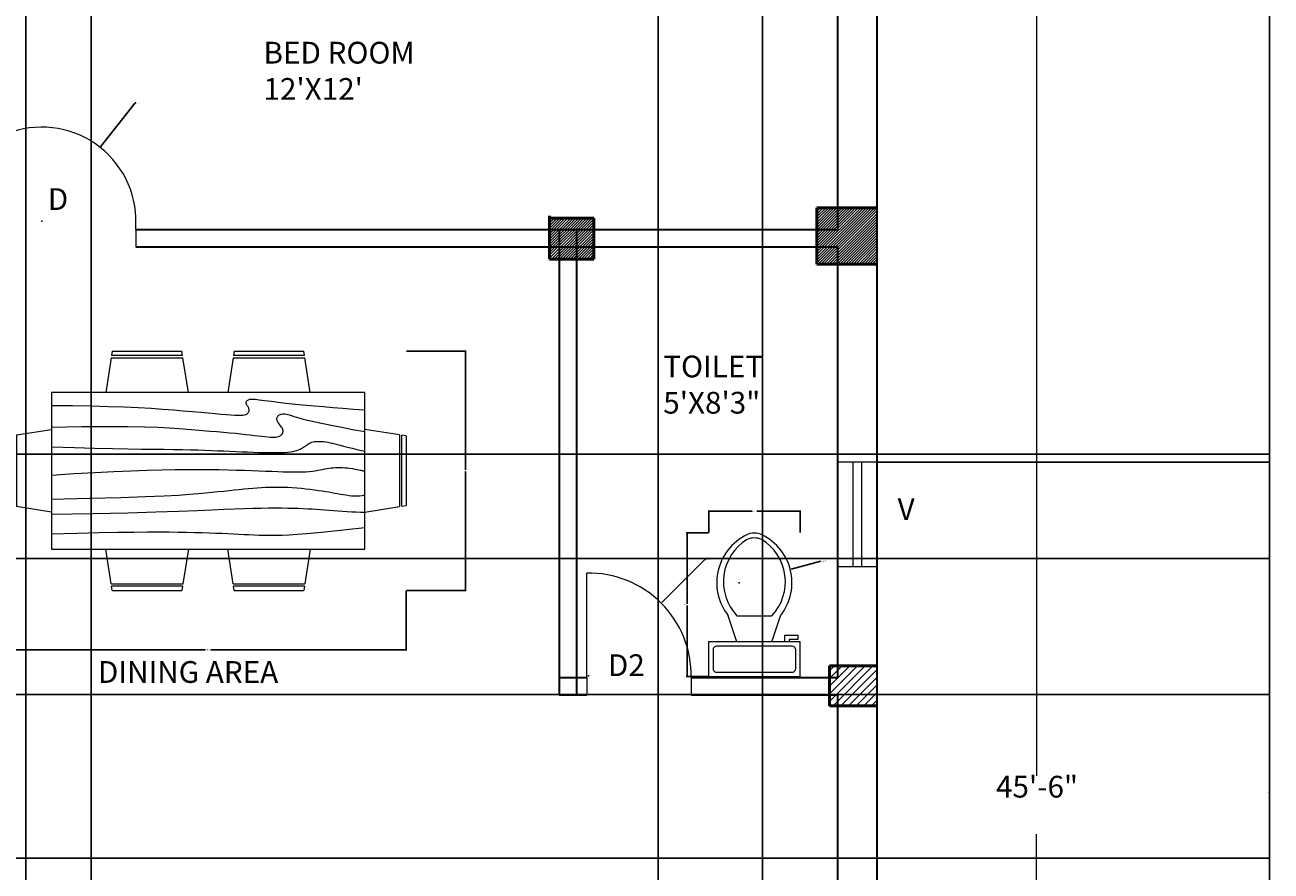
# Model space of a CAD drawing. Units: inches. Extents: x -12 to 472, y -585 to 99.
# Tile 3 of 4: x 186 to 472, y -281 to -86. Entities that reach past the tile are written whole.
import ezdxf

# ---------------------------------------------------------------- set-up
doc = ezdxf.new("R2010")
doc.units = ezdxf.units.IN
doc.header["$MEASUREMENT"] = 0
for name, color, linetype, lineweight in [('A-ANNO-DIMS', 2, 'Continuous', 18), ('A-ANNO-TEXT', 7, 'Continuous', 18), ('A-AREA-IDEN', 7, 'Continuous', 25), ('A-COLS', 7, 'Continuous', 50), ('A-COLS-PATT', 252, 'Continuous', 13), ('A-DOOR', 3, 'Continuous', 18), ('A-FLOR-FIXT', 9, 'Continuous', 20), ('A-FURN', 8, 'Continuous', 18), ('A-GLAZ', 4, 'Continuous', 18), ('A-WALL', 7, 'Continuous', 35)]:
    doc.layers.add(name, color=color, linetype=linetype, lineweight=lineweight)
doc.styles.get("Standard").update_dxf_attribs({"font": 'arial.ttf'})
doc.dimstyles.get("Standard").update_dxf_attribs({"dimtxt": 0.18, "dimasz": 0.18, "dimexe": 0.18, "dimexo": 0.0625, "dimgap": 0.09, "dimtad": 0, "dimtih": 1, "dimtoh": 1, "dimdec": 4, "dimzin": 0, "dimdsep": 46, "dimtxsty": 'Standard', "dimcen": 0.09, "dimadec": 0, "dimazin": 0, "dimtfac": 1, "dimtdec": 4, "dimtofl": 0, "dimtmove": 0, "dimatfit": 3, "dimfxl": 1, "dimtolj": 1, "dimtzin": 0, "dimarcsym": 0})

# ---------------------------------------------------------------- blocks, each defined once
blk = doc.blocks.new('Toilet - top')
for p, q in [((9.5, -6), (9.5, -2)), ((-10, -8.5), (-8, -8.5)), ((-10, -9.5), (-10, -8.5)), ((-8, -8.5), (-8, -8)), ((-7, -8), (-7, -9.5)), ((-4, -8), (-6, -14)), ((4, -8), (6, -14)), ((-7, -9.5), (-10, -9.5)), ((4, -14), (-4, -14))]:
    blk.add_line(p, q)
blk.add_lwpolyline([(10.5, -8), (10.5, 0), (-10.5, 0), (-10.5, -8)], close=True)
for points in [[(-9.5, -2), (-9.5, -6)], [(8.5, -1), (-8.5, -1)], [(-8.5, -7), (8.5, -7)]]:
    blk.add_lwpolyline(points)
for centre, radius, start, end in [((-8.62, -1.88), 0.884, 81.8699, 188.1301), ((8.62, -1.88), 0.884, 351.8699, 98.1301), ((-8.62, -6.12), 0.884, 171.8699, 278.1301), ((8.62, -6.12), 0.884, 261.8699, 8.1301), ((3.52, -21.58), 12.17, 141.4691, 247.9714), ((4.2, -21.82), 11.33, 136.3677, 238.9468), ((-3.52, -21.58), 12.17, 292.0284, 38.5307), ((-4.2, -21.82), 11.33, 301.053, 43.6321), ((0, -27.88), 4, 245.7318, 294.2682), ((0, -29), 4, 254.8605, 285.1395)]:
    blk.add_arc(centre, radius, start, end)
blk = doc.blocks.new('Dining Set - 36 x 72 in.')
for p, q in [((-22.2343, 26.00059), (-23.4847, 17.99762)), ((-22.2304, 26), (-5.7608, 26)), ((-22, 27.5), (-22.1562, 26.50042)), ((-5.8416, 26.5), (-22.1534, 26.5)), ((-22, 27.5), (-6, 27.5)), ((-5.8437, 26.49966), (-6, 27.5)), ((-4.5152, 17.99762), (-5.7655, 25.99926)), ((5.7657, 26.00059), (4.5153, 17.99762)), ((5.7696, 26), (22.2392, 26)), ((6, 27.5), (5.8438, 26.50042)), ((22.1584, 26.5), (5.8466, 26.5)), ((6, 27.5), (22, 27.5)), ((22.1563, 26.49966), (22, 27.5)), ((23.4848, 17.99762), (22.2345, 25.99926)), ((36, 18), (-36, 18)), ((-36, 18), (-36, -18)), ((36, -18), (36, 18)), ((-44.0006, 8.23428), (-35.9976, 9.48474)), ((44.0006, 8.23428), (35.9976, 9.48474)), ((-45.5, 8), (-44.5004, 8.15617)), ((-45.5, 8), (-45.5, -8)), ((-44.5, -8.15843), (-44.5, 8.15338)), ((-44, 8.23041), (-44, -8.23915)), ((44, 8.23041), (44, -8.23915)), ((44.5, -8.15843), (44.5, 8.15338)), ((45.5, 8), (44.5005, 8.15617)), ((45.5, 8), (45.5, -8)), ((-44.4997, -8.15631), (-45.5, -8)), ((-35.9976, -9.48476), (-43.9993, -8.2345)), ((35.9976, -9.48476), (43.9993, -8.2345)), ((44.4997, -8.15631), (45.5, -8)), ((-36, -18), (36, -18)), ((-22.2343, -26.0006), (-23.4847, -17.99762)), ((-4.5152, -17.99762), (-5.7655, -25.99928)), ((5.7657, -26.0006), (4.5153, -17.99762)), ((23.4848, -17.99762), (22.2345, -25.99928)), ((-22.2304, -26), (-5.7608, -26)), ((-22, -27.5), (-22.1562, -26.50044)), ((-5.8416, -26.5), (-22.1534, -26.5)), ((-22, -27.5), (-6, -27.5)), ((-5.8437, -26.49967), (-6, -27.5)), ((5.7696, -26), (22.2392, -26)), ((6, -27.5), (5.8438, -26.50044)), ((22.1584, -26.5), (5.8466, -26.5)), ((6, -27.5), (22, -27.5)), ((22.1563, -26.49967), (22, -27.5))]:
    blk.add_line(p, q)
for points in [[(-36, 15), (-31.1772, 14.97754), (-26.8079, 14.91406), (-22.8538, 14.81543), (-19.276, 14.6875), (-16.0362, 14.53613), (-13.0957, 14.36718), (-10.4159, 14.18652), (-7.9583, 14), (-5.6904, 13.81315), (-3.6035, 13.63021), (-1.6954, 13.45508), (0.0365, 13.29166), (1.5945, 13.14388), (2.9811, 13.01562), (4.1988, 12.9108), (5.25, 12.83333), (6.1393, 12.78613), (6.8802, 12.76823), (7.4883, 12.77767), (7.9792, 12.8125), (8.3685, 12.87077), (8.6719, 12.95052), (8.9049, 13.0498), (9.0833, 13.16666), (9.2205, 13.29899), (9.3216, 13.44401), (9.3895, 13.59879), (9.4271, 13.76041), (9.4373, 13.92594), (9.4232, 14.09245), (9.3875, 14.257), (9.3333, 14.41666), (9.2638, 14.56917), (9.1836, 14.71484), (9.0975, 14.85465), (9.0104, 14.98958), (8.9272, 15.1206), (8.8529, 15.2487), (8.7922, 15.37483), (8.75, 15.5), (8.7305, 15.62467), (8.7344, 15.74739), (8.7617, 15.86621), (8.8125, 15.97916), (8.8867, 16.08431), (8.9844, 16.17968), (9.1055, 16.26334), (9.25, 16.33333), (9.4189, 16.38802), (9.6172, 16.42708), (9.8506, 16.45052), (10.125, 16.45833), (10.4463, 16.45052), (10.8203, 16.42708), (11.2529, 16.38802), (11.75, 16.33333), (12.3184, 16.26318), (12.9694, 16.17838), (13.7151, 16.07991), (14.5677, 15.96875), (15.5395, 15.84586), (16.6426, 15.71224), (17.8893, 15.56884), (19.2917, 15.41666), (20.859, 15.25667), (22.5879, 15.08984), (24.4721, 14.91715), (26.5052, 14.73958), (28.6809, 14.5581), (30.9929, 14.3737), (33.4347, 14.18733), (36, 14)], [(-36, 10), (-28.9766, 10.14274), (-23.1725, 10.20442), (-18.4241, 10.19775), (-14.5677, 10.13541), (-11.4399, 10.03011), (-8.877, 9.89453), (-6.7154, 9.74137), (-4.7917, 9.58333), (-2.9698, 9.43082), (-1.2246, 9.28515), (0.4415, 9.14534), (2.026, 9.01041), (3.5266, 8.87939), (4.9408, 8.7513), (6.266, 8.62516), (7.5, 8.5), (8.6411, 8.37549), (9.6914, 8.2539), (10.6538, 8.13818), (11.5312, 8.03125), (12.3267, 7.93603), (13.043, 7.85547), (13.6831, 7.79248), (14.25, 7.75), (14.7471, 7.7303), (15.1797, 7.73307), (15.5537, 7.75732), (15.875, 7.80208), (16.1494, 7.86637), (16.3828, 7.94922), (16.5811, 8.04964), (16.75, 8.16666), (16.8944, 8.29915), (17.0143, 8.44531), (17.1089, 8.60319), (17.1771, 8.77083), (17.218, 8.94629), (17.2305, 9.1276), (17.2137, 9.31282), (17.1667, 9.5), (17.0895, 9.6875), (16.987, 9.875), (16.8649, 10.0625), (16.7292, 10.25), (16.5856, 10.4375), (16.4401, 10.625), (16.2985, 10.8125), (16.1667, 11), (16.05, 11.18733), (15.9518, 11.3737), (15.8752, 11.5581), (15.8229, 11.73958), (15.798, 11.91715), (15.8034, 12.08984), (15.842, 12.25667), (15.9167, 12.41666), (16.0295, 12.56836), (16.1784, 12.70833), (16.3605, 12.83268), (16.5729, 12.9375), (16.8127, 13.01888), (17.0768, 13.07291), (17.3625, 13.0957), (17.6667, 13.08333), (17.9894, 13.03312), (18.3418, 12.94726), (18.7382, 12.82918), (19.1927, 12.68229), (19.7195, 12.51001), (20.3327, 12.31575), (21.0465, 12.10294), (21.875, 11.875), (22.8357, 11.63354), (23.959, 11.37304), (25.2786, 11.08618), (26.8282, 10.76562), (28.6414, 10.40405), (30.752, 9.99414), (33.1936, 9.52856), (36, 9)], [(-36, 5.5), (-30.7157, 5.3348), (-26.069, 5.20963), (-21.9946, 5.11767), (-18.4271, 5.05208), (-15.3009, 5.00602), (-12.5508, 4.97265), (-10.1112, 4.94515), (-7.9167, 4.91666), (-5.909, 4.88167), (-4.0586, 4.83984), (-2.3429, 4.79215), (-0.7396, 4.73958), (0.7739, 4.6831), (2.22, 4.6237), (3.6213, 4.56233), (5, 4.5), (6.373, 4.43782), (7.7344, 4.3776), (9.0723, 4.32129), (10.375, 4.27083), (11.6309, 4.22819), (12.8281, 4.19531), (13.9551, 4.17415), (15, 4.16666), (15.954, 4.17448), (16.819, 4.19791), (17.6001, 4.23698), (18.3021, 4.29166), (18.9299, 4.36198), (19.4883, 4.44791), (19.9823, 4.54948), (20.4167, 4.66666), (20.7969, 4.79899), (21.1302, 4.94401), (21.4245, 5.09879), (21.6875, 5.26041), (21.9271, 5.42594), (22.1511, 5.59245), (22.3672, 5.757), (22.5834, 5.91666), (22.8065, 6.06868), (23.0404, 6.21093), (23.2879, 6.34147), (23.5521, 6.45833), (23.8358, 6.55957), (24.142, 6.64323), (24.4735, 6.70735), (24.8334, 6.75), (25.2235, 6.76969), (25.642, 6.76692), (26.0858, 6.74267), (26.5521, 6.69791), (27.0379, 6.63362), (27.5404, 6.55078), (28.0565, 6.45036), (28.5834, 6.33333), (29.1242, 6.19987), (29.7071, 6.04687), (30.3661, 5.87044), (31.1354, 5.66666), (32.0493, 5.43164), (33.142, 5.16146), (34.4475, 4.85221), (36, 4.5)], [(-36, -1), (-30.7915, -0.6591), (-26.0195, -0.38216), (-21.6519, -0.16284), (-17.6563, 0.00521), (-14.0005, 0.12833), (-10.6523, 0.21289), (-7.5796, 0.26522), (-4.75, 0.29166), (-2.134, 0.29793), (0.2878, 0.28711), (2.5317, 0.26163), (4.6146, 0.22396), (6.5529, 0.17651), (8.3633, 0.12174), (10.0623, 0.06209), (11.6667, 0), (13.1899, -0.06201), (14.6341, -0.1211), (15.9982, -0.17432), (17.2813, -0.21875), (18.4823, -0.25147), (19.6003, -0.26953), (20.6343, -0.27002), (21.5834, -0.25), (22.4481, -0.20768), (23.2357, -0.14584), (23.9549, -0.06836), (24.6146, 0.02083), (25.2235, 0.11784), (25.7904, 0.21875), (26.3241, 0.31966), (26.8334, 0.41666), (27.3265, 0.50618), (27.8099, 0.58593), (28.2894, 0.65397), (28.7709, 0.70833), (29.2601, 0.74707), (29.763, 0.76823), (30.2855, 0.76985), (30.8334, 0.75), (31.4088, 0.70784), (31.9994, 0.64713), (32.589, 0.57275), (33.1615, 0.48958), (33.7008, 0.4025), (34.1908, 0.3164), (34.6153, 0.23616), (34.9584, 0.16666), (35.2099, 0.11165), (35.3848, 0.07031), (35.504, 0.04069), (35.5886, 0.02083), (35.6594, 0.00879), (35.7377, 0.0026), (35.8442, 0.00032), (36, 0)], [(-36, -6.5), (-27.1843, -6.31267), (-20.084, -6.1263), (-14.469, -5.9419), (-10.1094, -5.76042), (-6.7752, -5.58285), (-4.2363, -5.41016), (-2.2629, -5.24333), (-0.625, -5.08334), (0.8708, -4.93099), (2.2715, -4.78646), (3.5872, -4.64974), (4.8281, -4.52084), (6.0046, -4.39974), (7.127, -4.28646), (8.2053, -4.18099), (9.25, -4.08334), (10.2705, -3.99382), (11.2734, -3.91407), (12.2647, -3.84603), (13.25, -3.79167), (14.2354, -3.75293), (15.2266, -3.73177), (16.2295, -3.73015), (17.25, -3.75), (18.2912, -3.79248), (19.3451, -3.85547), (20.4009, -3.93604), (21.4479, -4.03125), (22.4754, -4.13819), (23.4727, -4.25391), (24.4289, -4.37549), (25.3334, -4.5), (26.1785, -4.62492), (26.9694, -4.74935), (27.7145, -4.87281), (28.4219, -4.99479), (29.1, -5.11483), (29.7572, -5.23242), (30.4016, -5.34709), (31.0417, -5.45834), (31.6837, -5.56437), (32.3262, -5.65821), (32.9658, -5.73153), (33.599, -5.77604), (34.2224, -5.78345), (34.8327, -5.74545), (35.4264, -5.65373), (36, -5.5)], [(-36, -10), (-26.4022, -9.81299), (-18.4675, -9.62891), (-11.9839, -9.45069), (-6.7396, -9.28125), (-2.5226, -9.12354), (0.8789, -8.98047), (3.6769, -8.85498), (6.0833, -8.75), (8.2767, -8.66765), (10.3021, -8.60677), (12.1712, -8.56543), (13.8958, -8.54167), (15.4876, -8.53353), (16.9583, -8.53907), (18.3197, -8.55632), (19.5834, -8.58334), (20.7616, -8.61841), (21.8685, -8.66081), (22.9188, -8.71004), (23.9271, -8.76563), (24.9081, -8.82707), (25.8763, -8.89388), (26.8465, -8.96558), (27.8334, -9.04167), (28.8474, -9.12118), (29.8828, -9.20117), (30.93, -9.27824), (31.9792, -9.34896), (33.0205, -9.40991), (34.0443, -9.45768), (35.0407, -9.48885), (36, -9.5)], [(-36, -14.5), (-30.0881, -14.33513), (-25.0332, -14.21224), (-20.7312, -14.12647), (-17.0781, -14.07292), (-13.97, -14.04671), (-11.3027, -14.04297), (-8.9724, -14.05681), (-6.875, -14.08334), (-4.9224, -14.11833), (-3.0905, -14.16016), (-1.3709, -14.20785), (0.2448, -14.26042), (1.7647, -14.3169), (3.1973, -14.3763), (4.5507, -14.43767), (5.8333, -14.5), (7.0554, -14.5621), (8.235, -14.62175), (9.3922, -14.67652), (10.5469, -14.72396), (11.7192, -14.76164), (12.929, -14.78711), (14.1965, -14.79794), (15.5417, -14.79167), (16.9933, -14.76424), (18.6152, -14.70508), (20.4804, -14.60197), (22.6615, -14.44271), (25.2312, -14.21509), (28.2624, -13.9069), (31.8277, -13.50594), (36, -13)]]:
    blk.add_lwpolyline(points)
blk = doc.blocks.new('VENT-24IN-EXT')
for p, q in [((0, 5.5), (24, 5.5)), ((0, 3.5), (24, 3.5))]:
    blk.add_line(p, q)
blk.add_lwpolyline([(0, 9), (24, 9), (24, 0), (0, 0)], close=True)
blk = doc.blocks.new('*D20')
at = {"layer": 'A-ANNO-DIMS', "color": 0, "lineweight": -2, "transparency": 16777216}
for p, q in [((342.6, -203.13), (337.52, -203.13)), ((337.7, -203.31), (337.7, -219.47)), ((337.7, -236), (337.7, -219.84)), ((342.6, -236.18), (337.52, -236.18))]:
    blk.add_line(p, q, dxfattribs=at)
at = {"layer": 'A-ANNO-DIMS', "color": 0, "transparency": 16777216}
for points in [[(337.67, -203.31), (337.73, -203.31), (337.7, -203.13)], [(337.67, -236), (337.73, -236), (337.7, -236.18)]]:
    blk.add_solid(points, dxfattribs=at)
at = {"layer": 'Defpoints', "color": 0, "transparency": 16777216}
for p in [(342.66, -203.13), (337.7, -236.18), (342.66, -236.18)]:
    blk.add_point(p, dxfattribs=at)
at = {"layer": 'A-ANNO-DIMS', "color": 0, "transparency": 16777216, "insert": (337.7, -219.66), "char_height": 0.18, "attachment_point": 5}
blk.add_mtext('\\A1;WC 33 TYP.', dxfattribs=at)
blk = doc.blocks.new('*D21')
at = {"layer": 'A-ANNO-DIMS', "color": 0, "lineweight": -2, "transparency": 16777216}
for p, q in [((342.66, -203.07), (342.66, -198)), ((342.84, -198.18), (352.63, -198.18)), ((363.48, -198.18), (353.69, -198.18)), ((363.66, -203.07), (363.66, -198))]:
    blk.add_line(p, q, dxfattribs=at)
at = {"layer": 'A-ANNO-DIMS', "color": 0, "transparency": 16777216}
for points in [[(342.84, -198.15), (342.84, -198.21), (342.66, -198.18)], [(363.48, -198.15), (363.48, -198.21), (363.66, -198.18)]]:
    blk.add_solid(points, dxfattribs=at)
at = {"layer": 'Defpoints', "color": 0, "transparency": 16777216}
for p in [(342.66, -198.18), (342.66, -203.13), (363.66, -203.13)]:
    blk.add_point(p, dxfattribs=at)
at = {"layer": 'A-ANNO-DIMS', "color": 0, "transparency": 16777216, "insert": (353.16, -198.18), "char_height": 0.18, "attachment_point": 5}
blk.add_mtext('\\A1;21 TYP.', dxfattribs=at)
blk = doc.blocks.new('*D24')
at = {"layer": 'A-ANNO-DIMS', "color": 0, "lineweight": -2, "transparency": 16777216}
for p, q in [((182.14, -216.43), (182.14, -230.2)), ((273.14, -216.43), (273.14, -230.2)), ((182.32, -230.02), (226.97, -230.02)), ((272.96, -230.02), (228.31, -230.02))]:
    blk.add_line(p, q, dxfattribs=at)
at = {"layer": 'A-ANNO-DIMS', "color": 0, "transparency": 16777216}
for points in [[(182.32, -229.99), (182.32, -230.05), (182.14, -230.02)], [(272.96, -229.99), (272.96, -230.05), (273.14, -230.02)]]:
    blk.add_solid(points, dxfattribs=at)
at = {"layer": 'Defpoints', "color": 0, "transparency": 16777216}
for p in [(182.14, -216.37), (273.14, -216.37), (273.14, -230.02)]:
    blk.add_point(p, dxfattribs=at)
at = {"layer": 'A-ANNO-DIMS', "color": 0, "transparency": 16777216, "insert": (227.64, -230.02), "char_height": 0.18, "attachment_point": 5}
blk.add_mtext('\\A1;DINING 91', dxfattribs=at)
blk = doc.blocks.new('*D25')
at = {"layer": 'A-ANNO-DIMS', "color": 0, "lineweight": -2, "transparency": 16777216}
for p, q in [((273.2, -161.37), (286.97, -161.37)), ((286.79, -161.55), (286.79, -188.68)), ((286.79, -216.19), (286.79, -189.05)), ((273.2, -216.37), (286.97, -216.37))]:
    blk.add_line(p, q, dxfattribs=at)
at = {"layer": 'A-ANNO-DIMS', "color": 0, "transparency": 16777216}
for points in [[(286.76, -161.55), (286.82, -161.55), (286.79, -161.37)], [(286.76, -216.19), (286.82, -216.19), (286.79, -216.37)]]:
    blk.add_solid(points, dxfattribs=at)
at = {"layer": 'Defpoints', "color": 0, "transparency": 16777216}
for p in [(273.14, -161.37), (286.79, -161.37), (273.14, -216.37)]:
    blk.add_point(p, dxfattribs=at)
at = {"layer": 'A-ANNO-DIMS', "color": 0, "transparency": 16777216, "insert": (286.79, -188.87), "char_height": 0.18, "attachment_point": 5}
blk.add_mtext('\\A1;55', dxfattribs=at)
blk = doc.blocks.new('*D30')
at = {"layer": 'A-ANNO-DIMS', "color": 0, "lineweight": -2, "transparency": 16777216}
for p, q in [((185.8, -429.83), (185.8, 98.81)), ((185.98, 98.63), (193.09, 98.63)), ((200.62, 98.63), (193.51, 98.63)), ((200.8, -431.32), (200.8, 98.81))]:
    blk.add_line(p, q, dxfattribs=at)
at = {"layer": 'A-ANNO-DIMS', "color": 0, "transparency": 16777216}
for points in [[(185.98, 98.66), (185.98, 98.6), (185.8, 98.63)], [(200.62, 98.66), (200.62, 98.6), (200.8, 98.63)]]:
    blk.add_solid(points, dxfattribs=at)
at = {"layer": 'Defpoints', "color": 0, "transparency": 16777216}
for p in [(200.8, 98.63), (185.8, -429.9), (200.8, -431.38)]:
    blk.add_point(p, dxfattribs=at)
at = {"layer": 'A-ANNO-DIMS', "color": 0, "transparency": 16777216, "insert": (193.3, 98.63), "char_height": 0.18, "attachment_point": 5}
blk.add_mtext('\\A1;15', dxfattribs=at)
blk = doc.blocks.new('*D37')
at = {"layer": 'A-ANNO-DIMS', "color": 0, "lineweight": -2, "transparency": 16777216}
for p, q in [((138.68, -240.32), (471.69, -240.32)), ((471.51, -240.5), (471.51, -258.92)), ((471.51, -277.7), (471.51, -259.28)), ((138.68, -277.88), (471.69, -277.88))]:
    blk.add_line(p, q, dxfattribs=at)
at = {"layer": 'A-ANNO-DIMS', "color": 0, "transparency": 16777216}
for points in [[(471.48, -240.5), (471.54, -240.5), (471.51, -240.32)], [(471.48, -277.7), (471.54, -277.7), (471.51, -277.88)]]:
    blk.add_solid(points, dxfattribs=at)
at = {"layer": 'Defpoints', "color": 0, "transparency": 16777216}
for p in [(138.61, -240.32), (138.61, -277.88), (471.51, -277.88)]:
    blk.add_point(p, dxfattribs=at)
at = {"layer": 'A-ANNO-DIMS', "color": 0, "transparency": 16777216, "insert": (471.51, -259.1), "char_height": 0.18, "attachment_point": 5}
blk.add_mtext('\\A1;37.56', dxfattribs=at)
blk = doc.blocks.new('*D40')
at = {"layer": 'A-ANNO-DIMS', "color": 0, "lineweight": -2, "transparency": 16777216}
for p, q in [((331.04, -77.44), (331.04, -585.26)), ((355.04, -77.44), (355.04, -585.26)), ((331.22, -585.08), (342.82, -585.08)), ((354.86, -585.08), (343.26, -585.08))]:
    blk.add_line(p, q, dxfattribs=at)
at = {"layer": 'A-ANNO-DIMS', "color": 0, "transparency": 16777216}
for points in [[(331.22, -585.05), (331.22, -585.11), (331.04, -585.08)], [(354.86, -585.05), (354.86, -585.11), (355.04, -585.08)]]:
    blk.add_solid(points, dxfattribs=at)
at = {"layer": 'Defpoints', "color": 0, "transparency": 16777216}
for p in [(331.04, -77.38), (355.04, -77.38), (355.04, -585.08)]:
    blk.add_point(p, dxfattribs=at)
at = {"layer": 'A-ANNO-DIMS', "color": 0, "transparency": 16777216, "insert": (343.04, -585.08), "char_height": 0.18, "attachment_point": 5}
blk.add_mtext('\\A1;24', dxfattribs=at)
blk = doc.blocks.new('*D46')
at = {"layer": 'A-ANNO-DIMS', "color": 0, "lineweight": -2, "transparency": 16777216}
for p, q in [((133.34, -185.05), (471.69, -185.05)), ((471.51, -185.23), (471.51, -196.87)), ((471.51, -208.87), (471.51, -197.23)), ((133.34, -209.05), (471.69, -209.05))]:
    blk.add_line(p, q, dxfattribs=at)
at = {"layer": 'A-ANNO-DIMS', "color": 0, "transparency": 16777216}
for points in [[(471.48, -185.23), (471.54, -185.23), (471.51, -185.05)], [(471.48, -208.87), (471.54, -208.87), (471.51, -209.05)]]:
    blk.add_solid(points, dxfattribs=at)
at = {"layer": 'Defpoints', "color": 0, "transparency": 16777216}
for p in [(133.28, -185.05), (133.28, -209.05), (471.51, -209.05)]:
    blk.add_point(p, dxfattribs=at)
at = {"layer": 'A-ANNO-DIMS', "color": 0, "transparency": 16777216, "insert": (471.51, -197.05), "char_height": 0.18, "attachment_point": 5}
blk.add_mtext('\\A1;24', dxfattribs=at)
blk = doc.blocks.new('*D50')
at = {"layer": 'A-ANNO-DIMS', "color": 0, "lineweight": -2, "transparency": 16777216}
for p, q in [((381.34, 19.62), (471.69, 19.62)), ((471.51, 19.44), (471.51, -83.45)), ((471.51, -186.7), (471.51, -83.81)), ((381.34, -186.88), (471.69, -186.88))]:
    blk.add_line(p, q, dxfattribs=at)
at = {"layer": 'A-ANNO-DIMS', "color": 0, "transparency": 16777216}
for points in [[(471.48, 19.44), (471.54, 19.44), (471.51, 19.62)], [(471.48, -186.7), (471.54, -186.7), (471.51, -186.88)]]:
    blk.add_solid(points, dxfattribs=at)
at = {"layer": 'Defpoints', "color": 0, "transparency": 16777216}
for p in [(381.28, 19.62), (381.28, -186.88), (471.51, -186.88)]:
    blk.add_point(p, dxfattribs=at)
at = {"layer": 'A-ANNO-DIMS', "color": 0, "transparency": 16777216, "insert": (471.51, -83.63), "char_height": 0.18, "attachment_point": 5}
blk.add_mtext('\\A1;206.5', dxfattribs=at)
blk = doc.blocks.new('*D51')
at = {"layer": 'A-ANNO-DIMS', "color": 0, "lineweight": -2, "transparency": 16777216}
for p, q in [((381.34, -186.88), (471.69, -186.88)), ((471.51, -187.06), (471.51, -262.66)), ((471.51, -338.62), (471.51, -263.02)), ((381.34, -338.8), (471.69, -338.8))]:
    blk.add_line(p, q, dxfattribs=at)
at = {"layer": 'A-ANNO-DIMS', "color": 0, "transparency": 16777216}
for points in [[(471.48, -187.06), (471.54, -187.06), (471.51, -186.88)], [(471.48, -338.62), (471.54, -338.62), (471.51, -338.8)]]:
    blk.add_solid(points, dxfattribs=at)
at = {"layer": 'Defpoints', "color": 0, "transparency": 16777216}
for p in [(381.28, -186.88), (381.28, -338.8), (471.51, -338.8)]:
    blk.add_point(p, dxfattribs=at)
at = {"layer": 'A-ANNO-DIMS', "color": 0, "transparency": 16777216, "insert": (471.51, -262.84), "char_height": 0.18, "attachment_point": 5}
blk.add_mtext('\\A1;151.92', dxfattribs=at)
blk = doc.blocks.new('*D57')
at = {"layer": 'A-ANNO-DIMS', "color": 0, "lineweight": -2, "transparency": 16777216}
for p, q in [((341.76, -209.28), (331.87, -219.16)), ((341.94, -209.28), (341.76, -209.28)), ((314.98, -235.97), (315.16, -235.97)), ((315.07, -236.06), (315.07, -235.88))]:
    blk.add_line(p, q, dxfattribs=at)
at = {"layer": 'A-ANNO-DIMS', "color": 0, "transparency": 16777216}
blk.add_solid([(331.85, -219.14), (331.9, -219.18), (331.75, -219.28)], dxfattribs=at)
at = {"layer": 'Defpoints', "color": 0, "transparency": 16777216}
for p in [(331.75, -219.28), (315.07, -235.97)]:
    blk.add_point(p, dxfattribs=at)
at = {"layer": 'A-ANNO-DIMS', "color": 0, "transparency": 16777216, "insert": (342.42, -209.28), "char_height": 0.18, "attachment_point": 5}
blk.add_mtext('\\A1;R23.59', dxfattribs=at)
blk = doc.blocks.new('*D58')
at = {"layer": 'A-ANNO-DIMS', "color": 0, "lineweight": -2, "transparency": 16777216}
for p, q in [((210.88, -104.32), (202.95, -114.38)), ((211.06, -104.32), (210.88, -104.32)), ((189.35, -131.51), (189.53, -131.51)), ((189.44, -131.6), (189.44, -131.42))]:
    blk.add_line(p, q, dxfattribs=at)
at = {"layer": 'A-ANNO-DIMS', "color": 0, "transparency": 16777216}
blk.add_solid([(202.93, -114.36), (202.98, -114.39), (202.84, -114.52)], dxfattribs=at)
at = {"layer": 'Defpoints', "color": 0, "transparency": 16777216}
for p in [(202.84, -114.52), (189.44, -131.51)]:
    blk.add_point(p, dxfattribs=at)
at = {"layer": 'A-ANNO-DIMS', "color": 0, "transparency": 16777216, "insert": (211.61, -104.32), "char_height": 0.18, "attachment_point": 5}
blk.add_mtext('\\A1;R21.644', dxfattribs=at)
blk = doc.blocks.new('*D62')
at = {"layer": 'A-ANNO-DIMS', "color": 0, "lineweight": -2, "transparency": 16777216}
for p, q in [((368.47, -209.65), (361.58, -211.46)), ((349.55, -214.6), (349.73, -214.6)), ((349.64, -214.69), (349.64, -214.51))]:
    blk.add_line(p, q, dxfattribs=at)
at = {"layer": 'A-ANNO-DIMS', "color": 0, "transparency": 16777216}
blk.add_solid([(361.58, -211.43), (361.59, -211.49), (361.41, -211.51)], dxfattribs=at)
at = {"layer": 'Defpoints', "color": 0, "transparency": 16777216}
for p in [(361.41, -211.51), (349.64, -214.6)]:
    blk.add_point(p, dxfattribs=at)
at = {"layer": 'A-ANNO-DIMS', "color": 0, "transparency": 16777216, "insert": (369.15, -209.65), "char_height": 0.18, "attachment_point": 5}
blk.add_mtext('\\A1;4X R12.17', dxfattribs=at)

msp = doc.modelspace()

# ---------------------------------------------------------------- hatches: boundary and pattern name
at = {"layer": 'A-COLS-PATT'}
h = msp.add_hatch(dxfattribs=at)
h.set_pattern_fill('ANSI31', color=256, scale=3.5)
h.set_pattern_definition([(45, (-1281.90016, -702.76037), (-0.30935922, 0.30935922), [])])
h.paths.add_polyline_path([(178.2783, -133.3788), (174.2783, -133.3788), (174.2783, -137.3788), (178.2783, -137.3788)])
h.paths.add_polyline_path([(178.2783, -130.763), (174.2783, -130.763), (174.2783, -133.3788), (178.2783, -133.3788)])
h.paths.add_polyline_path([(174.2783, -130.763), (172.7504, -130.763), (172.7504, -133.3788), (174.2783, -133.3788)])
h.paths.add_polyline_path([(174.2783, -133.3788), (172.7504, -133.3788), (172.7504, -137.3788), (174.2783, -137.3788)])
h.paths.add_polyline_path([(181.0026, -137.3788), (172.7504, -137.3788), (172.7504, -139.195), (181.0026, -139.195)])
h.paths.add_polyline_path([(181.0026, -133.3788), (178.2783, -133.3788), (178.2783, -137.3788), (181.0026, -137.3788)])
h.paths.add_polyline_path([(181.0026, -130.763), (178.2783, -130.763), (178.2783, -133.3788), (181.0026, -133.3788)])
h.paths.add_polyline_path([(381.2783, -128.4288), (372.2783, -128.4288), (372.2783, -133.3788), (367.5282, -133.3788), (367.5282, -137.3788), (372.2783, -137.3788), (372.2783, -141.3418), (381.2783, -141.3418)])
h.paths.add_polyline_path([(372.2783, -128.4288), (367.5282, -128.4288), (367.5282, -133.3788), (372.2783, -133.3788)])
h.paths.add_polyline_path([(372.2783, -137.3788), (367.5282, -137.3788), (367.5282, -141.3418), (372.2783, -141.3418)], flags=17)
h.paths.add_polyline_path([(316.2734, -130.7939), (306.1194, -130.7939), (306.1194, -133.3788), (316.2734, -133.3788)])
h.paths.add_polyline_path([(312.2783, -133.3788), (308.2783, -133.3788), (308.2783, -137.3788), (312.2783, -137.3788)])
h.paths.add_polyline_path([(316.2734, -133.3788), (312.2783, -133.3788), (312.2783, -137.3788), (316.2734, -137.3788)])
h.paths.add_polyline_path([(316.2734, -137.3788), (312.2783, -137.3788), (312.2783, -140.1848), (316.2734, -140.1848)])
h.paths.add_polyline_path([(312.2783, -137.3788), (308.2783, -137.3788), (308.2783, -140.1848), (312.2783, -140.1848)])
h.paths.add_polyline_path([(308.2783, -137.3788), (306.1194, -137.3788), (306.1194, -140.1848), (308.2783, -140.1848)])
h.paths.add_polyline_path([(308.2783, -133.3788), (306.1194, -133.3788), (306.1194, -137.3788), (308.2783, -137.3788)])
h = msp.add_hatch(dxfattribs=at)
h.set_pattern_fill('ANSI31', color=256, scale=10)
h.set_pattern_definition([(45, (-1281.9002, -702.7604), (-0.8838835, 0.8838835), [])])
h.paths.add_polyline_path([(381.2783, -233.7271), (372.2783, -233.7271), (372.2783, -236.3788), (370.4204, -236.3788), (370.4204, -240.3788), (372.2783, -240.3788), (372.2783, -242.8621), (381.2783, -242.8621)])
h.paths.add_polyline_path([(372.2783, -233.7271), (370.4204, -233.7271), (370.4204, -236.3788), (372.2783, -236.3788)], flags=17)
h.paths.add_polyline_path([(372.2783, -240.3788), (370.4204, -240.3788), (370.4204, -242.8621), (372.2783, -242.8621)], flags=17)

# ---------------------------------------------------------------- linework, layer by layer
at = {"layer": 'A-ANNO-DIMS'}
for p, q in [((417.9974, 19.6212), (417.9974, -233.6801)), ((417.9974, -233.6801), (417.9974, -258.9855)), ((417.9974, -293.9965), (417.9974, -272.3584))]:
    msp.add_line(p, q, dxfattribs=at)
at = {"layer": 'A-COLS'}
for p, q in [((381.2783, -128.4288), (367.5282, -128.4288)), ((367.5282, -128.4288), (367.5282, -141.3418)), ((306.1194, -130.2305), (306.1194, -140.1848)), ((316.2734, -130.7939), (306.1194, -130.7939)), ((316.2734, -140.1848), (316.2734, -130.7939)), ((306.1194, -140.1848), (316.2734, -140.1848)), ((367.5282, -141.3418), (381.2783, -141.3418)), ((381.2783, -233.7271), (370.4204, -233.7271)), ((370.4204, -233.7271), (370.4204, -242.8621)), ((370.4204, -242.8621), (381.2783, -242.8621))]:
    msp.add_line(p, q, dxfattribs=at)
at = {"layer": 'A-DOOR'}
for p, q in [((211.0026, -133.3788), (211.0026, -137.3788)), ((314.6533, -236.3788), (314.6533, -212.3788)), ((314.6533, -236.3788), (314.6533, -240.3788)), ((338.6533, -236.3788), (338.6533, -240.3788))]:
    msp.add_line(p, q, dxfattribs=at)
for centre, radius, start, end in [((189.4395, -131.5126), 21.6437, 355.053745, 108.429724), ((315.0664, -235.9656), 23.5905, 358.996558, 91.003442)]:
    msp.add_arc(centre, radius, start, end, dxfattribs=at)
at = {"layer": 'A-WALL'}
for p, q in [((372.2783, -77.3788), (372.2783, -133.3788)), ((211.0026, -133.3788), (372.2783, -133.3788)), ((308.2783, -133.3788), (308.2783, -240.3788)), ((312.2783, -133.3788), (312.2783, -240.3788)), ((211.0026, -137.3788), (372.2783, -137.3788)), ((372.2783, -137.3788), (372.2783, -236.3788)), ((308.2783, -236.3788), (314.6533, -236.3788)), ((338.6533, -236.3788), (372.2783, -236.3788)), ((308.2783, -240.3788), (314.6533, -240.3788)), ((338.6533, -240.3788), (372.2783, -240.3788)), ((372.2783, -240.3788), (372.2783, -431.3788))]:
    msp.add_line(p, q, dxfattribs=at)
msp.add_lwpolyline([(21.2783, 19.6212), (381.2783, 19.6212), (381.2783, -526.3788), (21.2783, -526.3788)], close=True, dxfattribs=at)

# ---------------------------------------------------------------- block references
at = {"layer": 'A-FLOR-FIXT', "rotation": 180}
msp.add_blockref('Toilet - top', (353.1588, -236.1795), dxfattribs=at)
at = {"layer": 'A-FURN'}
msp.add_blockref('Dining Set - 36 x 72 in.', (227.6392, -188.8665), dxfattribs=at)
at = {"layer": 'A-GLAZ', "extrusion": (0, 0, -1), "zscale": -1, "rotation": 270.0000000000002}
msp.add_blockref('VENT-24IN-EXT', (-381.2785, -186.8789), dxfattribs=at)

# ---------------------------------------------------------------- texts
at = {"layer": 'A-ANNO-DIMS', "insert": (408.6762, -258.9855), "char_height": 5, "attachment_point": 1}
msp.add_mtext_dynamic_manual_height_columns('45\'-6"', width=68.171849, gutter_width=25, heights=[0], dxfattribs=at)
at = {"layer": 'A-ANNO-TEXT', "char_height": 5, "attachment_point": 1}
for s, width, insert in [('D', 16.174239, (190.8101, -123.9134)), ('V', 20.826633, (386.0703, -195.1789)), ('D2', 12.117402, (319.4998, -231.0503))]:
    msp.add_mtext_dynamic_manual_height_columns(s, width=width, gutter_width=25, heights=[0], dxfattribs=dict(at, insert=insert))
at = {"layer": 'A-AREA-IDEN', "char_height": 5, "attachment_point": 1}
for s, width, insert in [("BED ROOM\\P12'X12'", 104.621705, (240.3714, -90.2615)), ('TOILET\\P5\'X8\'3"', 55.538083, (332.2254, -162.3895)), ('DINING AREA', 97.088595, (202.3303, -232.6181))]:
    msp.add_mtext_dynamic_manual_height_columns(s, width=width, gutter_width=25, heights=[0], dxfattribs=dict(at, insert=insert))

# ---------------------------------------------------------------- dimensions: what is measured, and where the dimension line sits
at = {"layer": 'A-ANNO-DIMS'}
for base, p1, p2, picture, middle in [((200.803, 98.6273), (185.8034, -429.897), (200.803, -431.3788), '*D30', (193.3032, 98.6273)), ((355.0411, -585.0813), (331.0411, -77.3788), (355.0411, -77.3788), '*D40', (343.0411, -585.0813))]:
    dim = msp.add_linear_dim(base=base, p1=p1, p2=p2, dimstyle='Standard', override={"dimdec": 0, "dimlfac": 1, "dimrnd": 0, "dimzin": 0, "dimdsep": 46, "dimlunit": 2}, dxfattribs=at)
    dim.commit()
    dim.dimension.update_dxf_attribs({"geometry": picture, "text_midpoint": middle})
for base, p1, p2, override, picture, middle in [((471.5096, -186.8788), (381.2783, 19.6212), (381.2783, -186.8788), {"dimdec": 1, "dimlfac": 1, "dimrnd": 0, "dimzin": 0, "dimdsep": 46, "dimlunit": 2}, '*D50', (471.5096, -83.6288)), ((286.7892, -161.3665), (273.1392, -216.3665), (273.1392, -161.3665), {"dimdec": 0, "dimlfac": 1, "dimrnd": 0, "dimzin": 0, "dimdsep": 46, "dimlunit": 2}, '*D25', (286.7892, -188.8665)), ((471.5096, -209.0467), (133.2783, -185.0467), (133.2783, -209.0467), {"dimdec": 0, "dimlfac": 1, "dimrnd": 0, "dimzin": 0, "dimdsep": 46, "dimlunit": 2}, '*D46', (471.5096, -197.0467)), ((471.5096, -338.8003), (381.2783, -186.8788), (381.2783, -338.8003), {"dimdec": 2, "dimlfac": 1, "dimrnd": 0, "dimzin": 0, "dimdsep": 46, "dimlunit": 2}, '*D51', (471.5096, -262.8395)), ((471.5096, -277.8788), (138.6133, -240.3222), (138.6133, -277.8788), {"dimdec": 2, "dimlfac": 1, "dimrnd": 0, "dimzin": 0, "dimdsep": 46, "dimlunit": 2}, '*D37', (471.5096, -259.1005))]:
    dim = msp.add_linear_dim(base=base, p1=p1, p2=p2, angle=90, dimstyle='Standard', override=override, dxfattribs=at)
    dim.commit()
    dim.dimension.update_dxf_attribs({"geometry": picture, "text_midpoint": middle})
for center, mpoint, override, picture, middle in [((189.4395, -131.5126), (202.841, -114.517), {"dimdec": 3, "dimlfac": 1, "dimrnd": 0, "dimzin": 0, "dimdsep": 46, "dimlunit": 2}, '*D58', (211.6112, -104.3197)), ((315.0664, -235.9656), (331.7474, -219.2846), {"dimdec": 2, "dimlfac": 1, "dimrnd": 0, "dimzin": 0, "dimdsep": 46, "dimlunit": 2}, '*D57', (342.416, -209.276))]:
    dim = msp.add_radius_dim(center=center, mpoint=mpoint, dimstyle='Standard', override=override, dxfattribs=at)
    dim.commit()
    dim.dimension.update_dxf_attribs({"geometry": picture, "text_midpoint": middle, "dimtype": 164})
for base, p1, p2, angle, text, picture, middle in [((342.6588, -198.1764), (363.6588, -203.1333), (342.6588, -203.1333), 180, '<> TYP.', '*D21', (353.1588, -198.1764)), ((337.7019, -236.1795), (342.6588, -203.1333), (342.6588, -236.1795), 270, 'WC <> TYP.', '*D20', (337.7019, -219.6564))]:
    dim = msp.add_linear_dim(base=base, p1=p1, p2=p2, angle=angle, text=text, dimstyle='Standard', override={"dimdec": 0, "dimlfac": 1, "dimrnd": 0, "dimzin": 0, "dimdsep": 46, "dimlunit": 2}, dxfattribs=at)
    dim.commit()
    dim.dimension.update_dxf_attribs({"geometry": picture, "text_midpoint": middle})
dim = msp.add_radius_dim(center=(349.6392, -214.599), mpoint=(361.4089, -211.507), text='4X <>', dimstyle='Standard', override={"dimdec": 2, "dimlfac": 1, "dimrnd": 0, "dimzin": 0, "dimdsep": 46, "dimlunit": 2}, dxfattribs=at)
dim.commit()
dim.dimension.update_dxf_attribs({"geometry": '*D62', "text_midpoint": (368.4707, -209.6518), "dimtype": 164})
dim = msp.add_linear_dim(base=(273.1392, -230.0165), p1=(182.1392, -216.3665), p2=(273.1392, -216.3665), text='DINING <>', dimstyle='Standard', override={"dimdec": 0, "dimlfac": 1, "dimrnd": 0, "dimzin": 0, "dimdsep": 46, "dimlunit": 2}, dxfattribs=at)
dim.commit()
dim.dimension.update_dxf_attribs({"geometry": '*D24', "text_midpoint": (227.6392, -230.0165)})

doc.saveas('drawing.dxf')
